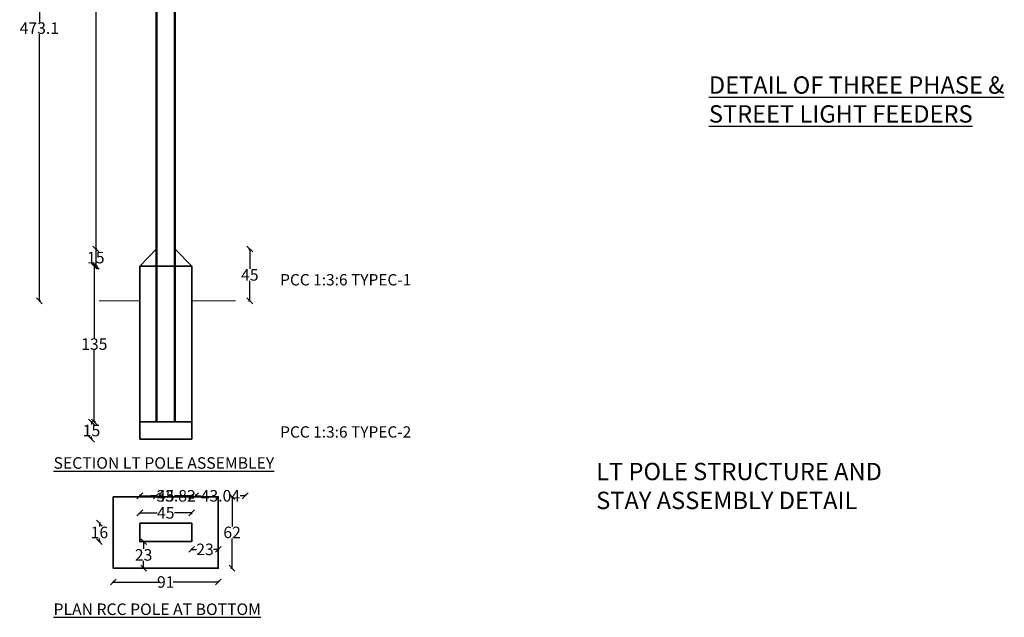
# Model space of a CAD drawing. Units: centimetres. Extents: x -70 to 1009, y -133 to 977.
# Tile 1 of 3: x -66 to 787, y -133 to 385. Entities that reach past the tile are written whole.
import ezdxf

# ---------------------------------------------------------------- set-up
doc = ezdxf.new("R2010")
doc.units = ezdxf.units.CM
doc.header["$MEASUREMENT"] = 0
for name, color, linetype, lineweight in [('C-TOPO', 8, 'Continuous', 18), ('E-ANNO-DIMS', 2, 'Continuous', 18), ('E-ANNO-TEXT', 7, 'Continuous', 25), ('E-POLE', 7, 'Continuous', 50), ('S-FNDN', 1, 'Continuous', 35)]:
    doc.layers.add(name, color=color, linetype=linetype, lineweight=lineweight)
doc.styles.get("Standard").update_dxf_attribs({"font": 'arial.ttf'})
doc.dimstyles.get("Standard").update_dxf_attribs({"dimtxt": 10, "dimasz": 5, "dimexe": 0.1, "dimexo": 0.1, "dimgap": 0.09, "dimtad": 0, "dimtih": 1, "dimtoh": 1, "dimdec": 0, "dimzin": 0, "dimdsep": 46, "dimtxsty": 'Standard', "dimblk": 'OBLIQUE', "dimcen": 0.09, "dimadec": 0, "dimazin": 0, "dimtfac": 1, "dimtdec": 0, "dimtofl": 0, "dimtmove": 0, "dimatfit": 3, "dimfxl": 1, "dimfxlon": 1, "dimtolj": 1, "dimtzin": 0, "dimarcsym": 0})

# ---------------------------------------------------------------- blocks, each defined once
blk = doc.blocks.new('_Oblique')
at = {"color": 0, "linetype": 'ByBlock', "lineweight": -2}
blk.add_line((-0.5, -0.5), (0.5, 0.5), dxfattribs=at)
blk = doc.blocks.new('*D3')
at = {"layer": 'Defpoints', "color": 0, "transparency": 16777216}
for p in [(52.24, 921.22), (-0.04, 171.22), (52.24, 171.22)]:
    blk.add_point(p, dxfattribs=at)
at = {"layer": 'E-ANNO-DIMS', "color": 0, "lineweight": -2, "transparency": 16777216}
for p, q in [((0.96, 921.22), (-0.14, 921.22)), ((-0.04, 921.22), (-0.04, 551.41)), ((-0.04, 171.22), (-0.04, 541.02)), ((0.96, 171.22), (-0.14, 171.22))]:
    blk.add_line(p, q, dxfattribs=at)
at = {"layer": 'E-ANNO-DIMS', "color": 0, "lineweight": -2, "transparency": 16777216, "xscale": 5, "yscale": 5, "zscale": 5}
for p, rotation in [((-0.04, 921.22), 90), ((-0.04, 171.22), 270)]:
    blk.add_blockref('_Oblique', p, dxfattribs=dict(at, rotation=rotation))
at = {"layer": 'E-ANNO-DIMS', "color": 0, "transparency": 16777216, "insert": (-0.04, 546.22), "char_height": 10, "attachment_point": 5}
blk.add_mtext('\\A1;750', dxfattribs=at)
blk = doc.blocks.new('*D4')
at = {"layer": 'Defpoints', "color": 0, "transparency": 16777216}
for p in [(-0.42, 186.22), (52.24, 186.22), (52.75, 171.22)]:
    blk.add_point(p, dxfattribs=at)
at = {"layer": 'E-ANNO-DIMS', "color": 0, "lineweight": -2, "transparency": 16777216}
for p, q in [((0.58, 186.22), (-0.52, 186.22)), ((-0.42, 186.22), (-0.42, 183.91)), ((0.58, 171.22), (-0.52, 171.22)), ((-0.42, 171.22), (-0.42, 173.52))]:
    blk.add_line(p, q, dxfattribs=at)
at = {"layer": 'E-ANNO-DIMS', "color": 0, "lineweight": -2, "transparency": 16777216, "xscale": 5, "yscale": 5, "zscale": 5}
for p, rotation in [((-0.42, 186.22), 90), ((-0.42, 171.22), 270)]:
    blk.add_blockref('_Oblique', p, dxfattribs=dict(at, rotation=rotation))
at = {"layer": 'E-ANNO-DIMS', "color": 0, "transparency": 16777216, "insert": (-0.42, 178.72), "char_height": 10, "attachment_point": 5}
blk.add_mtext('\\A1;15', dxfattribs=at)
blk = doc.blocks.new('*D5')
at = {"layer": 'Defpoints', "color": 0, "transparency": 16777216}
for p in [(37.74, 171.22), (-1.69, 36.22), (37.74, 36.22)]:
    blk.add_point(p, dxfattribs=at)
at = {"layer": 'E-ANNO-DIMS', "color": 0, "lineweight": -2, "transparency": 16777216}
for p, q in [((-0.69, 171.22), (-1.79, 171.22)), ((-1.69, 171.22), (-1.69, 108.91)), ((-1.69, 36.22), (-1.69, 98.52)), ((-0.69, 36.22), (-1.79, 36.22))]:
    blk.add_line(p, q, dxfattribs=at)
at = {"layer": 'E-ANNO-DIMS', "color": 0, "lineweight": -2, "transparency": 16777216, "xscale": 5, "yscale": 5, "zscale": 5}
for p, rotation in [((-1.69, 171.22), 90), ((-1.69, 36.22), 270)]:
    blk.add_blockref('_Oblique', p, dxfattribs=dict(at, rotation=rotation))
at = {"layer": 'E-ANNO-DIMS', "color": 0, "transparency": 16777216, "insert": (-1.69, 103.72), "char_height": 10, "attachment_point": 5}
blk.add_mtext('\\A1;135', dxfattribs=at)
blk = doc.blocks.new('*D6')
at = {"layer": 'Defpoints', "color": 0, "transparency": 16777216}
for p in [(37.74, 36.22), (-4.14, 21.22), (37.74, 21.22)]:
    blk.add_point(p, dxfattribs=at)
at = {"layer": 'E-ANNO-DIMS', "color": 0, "lineweight": -2, "transparency": 16777216}
for p, q in [((-3.14, 36.22), (-4.24, 36.22)), ((-4.14, 36.22), (-4.14, 33.91)), ((-3.14, 21.22), (-4.24, 21.22)), ((-4.14, 21.22), (-4.14, 23.52))]:
    blk.add_line(p, q, dxfattribs=at)
at = {"layer": 'E-ANNO-DIMS', "color": 0, "lineweight": -2, "transparency": 16777216, "xscale": 5, "yscale": 5, "zscale": 5}
for p, rotation in [((-4.14, 36.22), 90), ((-4.14, 21.22), 270)]:
    blk.add_blockref('_Oblique', p, dxfattribs=dict(at, rotation=rotation))
at = {"layer": 'E-ANNO-DIMS', "color": 0, "transparency": 16777216, "insert": (-4.14, 28.72), "char_height": 10, "attachment_point": 5}
blk.add_mtext('\\A1;15', dxfattribs=at)
blk = doc.blocks.new('*D7')
at = {"layer": 'Defpoints', "color": 0, "transparency": 16777216}
for p in [(68.24, 186.22), (133.11, 186.22), (68.24, 141.22)]:
    blk.add_point(p, dxfattribs=at)
at = {"layer": 'E-ANNO-DIMS', "color": 0, "lineweight": -2, "transparency": 16777216}
for p, q in [((132.11, 186.22), (133.21, 186.22)), ((133.11, 186.22), (133.11, 168.89)), ((133.11, 141.22), (133.11, 158.54)), ((132.11, 141.22), (133.21, 141.22))]:
    blk.add_line(p, q, dxfattribs=at)
at = {"layer": 'E-ANNO-DIMS', "color": 0, "lineweight": -2, "transparency": 16777216, "xscale": 5, "yscale": 5, "zscale": 5}
for p, rotation in [((133.11, 186.22), 90), ((133.11, 141.22), 270)]:
    blk.add_blockref('_Oblique', p, dxfattribs=dict(at, rotation=rotation))
at = {"layer": 'E-ANNO-DIMS', "color": 0, "transparency": 16777216, "insert": (133.11, 163.72), "char_height": 10, "attachment_point": 5}
blk.add_mtext('\\A1;45', dxfattribs=at)
blk = doc.blocks.new('*D8')
at = {"layer": 'Defpoints', "color": 0, "transparency": 16777216}
for p in [(82.74, -42.66), (37.74, -51.63), (82.74, -51.63)]:
    blk.add_point(p, dxfattribs=at)
at = {"layer": 'E-ANNO-DIMS', "color": 0, "lineweight": -2, "transparency": 16777216}
for p, q in [((37.74, -43.66), (37.74, -42.56)), ((37.74, -42.66), (52.75, -42.66)), ((82.74, -42.66), (67.73, -42.66)), ((82.74, -43.66), (82.74, -42.56))]:
    blk.add_line(p, q, dxfattribs=at)
at = {"layer": 'E-ANNO-DIMS', "color": 0, "lineweight": -2, "transparency": 16777216, "xscale": 5, "yscale": 5, "zscale": 5, "rotation": 180}
blk.add_blockref('_Oblique', (37.74, -42.66), dxfattribs=at)
at = {"layer": 'E-ANNO-DIMS', "color": 0, "lineweight": -2, "transparency": 16777216, "xscale": 5, "yscale": 5, "zscale": 5}
blk.add_blockref('_Oblique', (82.74, -42.66), dxfattribs=at)
at = {"layer": 'E-ANNO-DIMS', "color": 0, "transparency": 16777216, "insert": (60.24, -42.66), "char_height": 10, "attachment_point": 5}
blk.add_mtext('\\A1;45', dxfattribs=at)
blk = doc.blocks.new('*D9')
at = {"layer": 'Defpoints', "color": 0, "transparency": 16777216}
for p in [(82.74, -67.63), (105.74, -67.63), (105.74, -74.34)]:
    blk.add_point(p, dxfattribs=at)
at = {"layer": 'E-ANNO-DIMS', "color": 0, "lineweight": -2, "transparency": 16777216}
for p, q in [((82.74, -73.34), (82.74, -74.44)), ((82.74, -74.34), (86.9, -74.34)), ((105.74, -74.34), (101.58, -74.34)), ((105.74, -73.34), (105.74, -74.44))]:
    blk.add_line(p, q, dxfattribs=at)
at = {"layer": 'E-ANNO-DIMS', "color": 0, "lineweight": -2, "transparency": 16777216, "xscale": 5, "yscale": 5, "zscale": 5, "rotation": 180}
blk.add_blockref('_Oblique', (82.74, -74.34), dxfattribs=at)
at = {"layer": 'E-ANNO-DIMS', "color": 0, "lineweight": -2, "transparency": 16777216, "xscale": 5, "yscale": 5, "zscale": 5}
blk.add_blockref('_Oblique', (105.74, -74.34), dxfattribs=at)
at = {"layer": 'E-ANNO-DIMS', "color": 0, "transparency": 16777216, "insert": (94.24, -74.34), "char_height": 10, "attachment_point": 5}
blk.add_mtext('\\A1;23', dxfattribs=at)
blk = doc.blocks.new('*D10')
at = {"layer": 'Defpoints', "color": 0, "transparency": 16777216}
for p in [(37.74, -67.63), (37.74, -90.63), (41.03, -90.63)]:
    blk.add_point(p, dxfattribs=at)
at = {"layer": 'E-ANNO-DIMS', "color": 0, "lineweight": -2, "transparency": 16777216}
for p, q in [((40.03, -67.63), (41.13, -67.63)), ((41.03, -67.63), (41.03, -73.93)), ((41.03, -90.63), (41.03, -84.33)), ((40.03, -90.63), (41.13, -90.63))]:
    blk.add_line(p, q, dxfattribs=at)
at = {"layer": 'E-ANNO-DIMS', "color": 0, "lineweight": -2, "transparency": 16777216, "xscale": 5, "yscale": 5, "zscale": 5}
for p, rotation in [((41.03, -67.63), 90), ((41.03, -90.63), 270)]:
    blk.add_blockref('_Oblique', p, dxfattribs=dict(at, rotation=rotation))
at = {"layer": 'E-ANNO-DIMS', "color": 0, "transparency": 16777216, "insert": (41.03, -79.13), "char_height": 10, "attachment_point": 5}
blk.add_mtext('\\A1;23', dxfattribs=at)
blk = doc.blocks.new('*D21')
at = {"layer": 'Defpoints', "color": 0, "transparency": 16777216}
for p in [(14.74, -90.63), (105.74, -90.63), (105.74, -102.63)]:
    blk.add_point(p, dxfattribs=at)
at = {"layer": 'E-ANNO-DIMS', "color": 0, "lineweight": -2, "transparency": 16777216}
for p, q in [((14.74, -101.63), (14.74, -102.73)), ((105.74, -101.63), (105.74, -102.73)), ((14.74, -102.63), (53.95, -102.63)), ((105.74, -102.63), (66.53, -102.63))]:
    blk.add_line(p, q, dxfattribs=at)
at = {"layer": 'E-ANNO-DIMS', "color": 0, "lineweight": -2, "transparency": 16777216, "xscale": 5, "yscale": 5, "zscale": 5, "rotation": 180}
blk.add_blockref('_Oblique', (14.74, -102.63), dxfattribs=at)
at = {"layer": 'E-ANNO-DIMS', "color": 0, "lineweight": -2, "transparency": 16777216, "xscale": 5, "yscale": 5, "zscale": 5}
blk.add_blockref('_Oblique', (105.74, -102.63), dxfattribs=at)
at = {"layer": 'E-ANNO-DIMS', "color": 0, "transparency": 16777216, "insert": (60.24, -102.63), "char_height": 10, "attachment_point": 5}
blk.add_mtext('\\A1;91', dxfattribs=at)
blk = doc.blocks.new('*D22')
at = {"layer": 'Defpoints', "color": 0, "transparency": 16777216}
for p in [(105.74, -28.63), (117.74, -28.63), (105.74, -90.63)]:
    blk.add_point(p, dxfattribs=at)
at = {"layer": 'E-ANNO-DIMS', "color": 0, "lineweight": -2, "transparency": 16777216}
for p, q in [((116.74, -28.63), (117.84, -28.63)), ((117.74, -28.63), (117.74, -54.44)), ((117.74, -90.63), (117.74, -64.83)), ((116.74, -90.63), (117.84, -90.63))]:
    blk.add_line(p, q, dxfattribs=at)
at = {"layer": 'E-ANNO-DIMS', "color": 0, "lineweight": -2, "transparency": 16777216, "xscale": 5, "yscale": 5, "zscale": 5}
for p, rotation in [((117.74, -28.63), 90), ((117.74, -90.63), 270)]:
    blk.add_blockref('_Oblique', p, dxfattribs=dict(at, rotation=rotation))
at = {"layer": 'E-ANNO-DIMS', "color": 0, "transparency": 16777216, "insert": (117.74, -59.63), "char_height": 10, "attachment_point": 5}
blk.add_mtext('\\A1;62', dxfattribs=at)
blk = doc.blocks.new('*D23')
at = {"layer": 'Defpoints', "color": 0, "transparency": 16777216}
for p in [(2.74, -51.63), (37.74, -51.63), (37.74, -67.63)]:
    blk.add_point(p, dxfattribs=at)
at = {"layer": 'E-ANNO-DIMS', "color": 0, "lineweight": -2, "transparency": 16777216}
for p, q in [((3.74, -51.63), (2.64, -51.63)), ((2.74, -51.63), (2.74, -54.44)), ((3.74, -67.63), (2.64, -67.63)), ((2.74, -67.63), (2.74, -64.83))]:
    blk.add_line(p, q, dxfattribs=at)
at = {"layer": 'E-ANNO-DIMS', "color": 0, "lineweight": -2, "transparency": 16777216, "xscale": 5, "yscale": 5, "zscale": 5}
for p, rotation in [((2.74, -51.63), 90), ((2.74, -67.63), 270)]:
    blk.add_blockref('_Oblique', p, dxfattribs=dict(at, rotation=rotation))
at = {"layer": 'E-ANNO-DIMS', "color": 0, "transparency": 16777216, "insert": (2.74, -59.63), "char_height": 10, "attachment_point": 5}
blk.add_mtext('\\A1;16', dxfattribs=at)
blk = doc.blocks.new('*D25')
at = {"layer": 'Defpoints', "color": 0, "transparency": 16777216}
for p in [(37.74, 21.22), (82.74, 21.22), (82.74, -27.88)]:
    blk.add_point(p, dxfattribs=at)
at = {"layer": 'E-ANNO-DIMS', "color": 0, "lineweight": -2, "transparency": 16777216}
for p, q in [((37.74, -26.88), (37.74, -27.98)), ((37.74, -27.88), (52.75, -27.88)), ((82.74, -27.88), (67.73, -27.88)), ((82.74, -26.88), (82.74, -27.98))]:
    blk.add_line(p, q, dxfattribs=at)
at = {"layer": 'E-ANNO-DIMS', "color": 0, "lineweight": -2, "transparency": 16777216, "xscale": 5, "yscale": 5, "zscale": 5, "rotation": 180}
blk.add_blockref('_Oblique', (37.74, -27.88), dxfattribs=at)
at = {"layer": 'E-ANNO-DIMS', "color": 0, "lineweight": -2, "transparency": 16777216, "xscale": 5, "yscale": 5, "zscale": 5}
blk.add_blockref('_Oblique', (82.74, -27.88), dxfattribs=at)
at = {"layer": 'E-ANNO-DIMS', "color": 0, "transparency": 16777216, "insert": (60.24, -27.88), "char_height": 10, "attachment_point": 5}
blk.add_mtext('\\A1;45', dxfattribs=at)
blk = doc.blocks.new('*D34')
at = {"layer": 'Defpoints', "color": 0, "transparency": 16777216}
for p in [(52.24, 614.28), (-49.36, 141.22), (2.39, 141.22)]:
    blk.add_point(p, dxfattribs=at)
at = {"layer": 'E-ANNO-DIMS', "color": 0, "lineweight": -2, "transparency": 16777216}
for p, q in [((-48.36, 614.28), (-49.46, 614.28)), ((-49.36, 614.28), (-49.36, 382.95)), ((-49.36, 141.22), (-49.36, 372.55)), ((-48.36, 141.22), (-49.46, 141.22))]:
    blk.add_line(p, q, dxfattribs=at)
at = {"layer": 'E-ANNO-DIMS', "color": 0, "lineweight": -2, "transparency": 16777216, "xscale": 5, "yscale": 5, "zscale": 5}
for p, rotation in [((-49.36, 614.28), 90), ((-49.36, 141.22), 270)]:
    blk.add_blockref('_Oblique', p, dxfattribs=dict(at, rotation=rotation))
at = {"layer": 'E-ANNO-DIMS', "color": 0, "transparency": 16777216, "insert": (-49.36, 377.75), "char_height": 10, "attachment_point": 5}
blk.add_mtext('\\A1;473.1', dxfattribs=at)
blk = doc.blocks.new('*D35')
at = {"layer": 'Defpoints', "color": 0, "transparency": 16777216}
for p in [(52.23894, 639.625874), (86.058746, 612.513226), (86.058746, -27.884542)]:
    blk.add_point(p, dxfattribs=at)
at = {"layer": 'E-ANNO-DIMS', "color": 0, "lineweight": -2, "transparency": 16777216}
for p, q in [((52.23894, -27.884542), (47.23894, -27.884542)), ((52.23894, -26.884542), (52.23894, -27.984542)), ((86.058746, -26.884542), (86.058746, -27.984542)), ((86.058746, -27.884542), (91.058746, -27.884542))]:
    blk.add_line(p, q, dxfattribs=at)
at = {"layer": 'E-ANNO-DIMS', "color": 0, "lineweight": -2, "transparency": 16777216, "xscale": 5, "yscale": 5, "zscale": 5}
blk.add_blockref('_Oblique', (52.23894, -27.884542), dxfattribs=at)
at = {"layer": 'E-ANNO-DIMS', "color": 0, "lineweight": -2, "transparency": 16777216, "xscale": 5, "yscale": 5, "zscale": 5, "rotation": 180}
blk.add_blockref('_Oblique', (86.058746, -27.884542), dxfattribs=at)
at = {"layer": 'E-ANNO-DIMS', "color": 0, "transparency": 16777216, "insert": (69.148843, -27.884542), "char_height": 10, "attachment_point": 5}
blk.add_mtext('\\A1;33.82', dxfattribs=at)
blk = doc.blocks.new('*D36')
at = {"layer": 'Defpoints', "color": 0, "transparency": 16777216}
for p in [(129.1, 671.11), (86.06, 612.51), (129.1, -27.88)]:
    blk.add_point(p, dxfattribs=at)
at = {"layer": 'E-ANNO-DIMS', "color": 0, "lineweight": -2, "transparency": 16777216}
for p, q in [((86.06, -26.88), (86.06, -27.98)), ((86.06, -27.88), (90.43, -27.88)), ((129.1, -27.88), (124.72, -27.88)), ((129.1, -26.88), (129.1, -27.98))]:
    blk.add_line(p, q, dxfattribs=at)
at = {"layer": 'E-ANNO-DIMS', "color": 0, "lineweight": -2, "transparency": 16777216, "xscale": 5, "yscale": 5, "zscale": 5, "rotation": 180}
blk.add_blockref('_Oblique', (86.06, -27.88), dxfattribs=at)
at = {"layer": 'E-ANNO-DIMS', "color": 0, "lineweight": -2, "transparency": 16777216, "xscale": 5, "yscale": 5, "zscale": 5}
blk.add_blockref('_Oblique', (129.1, -27.88), dxfattribs=at)
at = {"layer": 'E-ANNO-DIMS', "color": 0, "transparency": 16777216, "insert": (107.58, -27.88), "char_height": 10, "attachment_point": 5}
blk.add_mtext('\\A1;43.04', dxfattribs=at)

msp = doc.modelspace()

# ---------------------------------------------------------------- linework, layer by layer
at = {"layer": 'C-TOPO'}
for p, q in [((37.7389, 141.2155), (2.3883, 141.2155)), ((82.7389, 141.2155), (120.6906, 141.2155))]:
    msp.add_line(p, q, dxfattribs=at)
at = {"layer": 'E-POLE'}
for p, q in [((52.2389, 171.2155), (52.2389, 921.2155)), ((68.2389, 171.2155), (68.2389, 921.2155)), ((68.2389, 186.2155), (68.2389, 141.2155)), ((52.2389, 36.2155), (52.2389, 171.2155)), ((68.2389, 36.2155), (68.2389, 171.2155))]:
    msp.add_line(p, q, dxfattribs=at)
at = {"layer": 'S-FNDN'}
for p, q in [((52.2389, 186.2155), (37.7389, 171.2155)), ((68.2389, 186.2155), (82.7389, 171.2155)), ((82.7389, 171.2155), (37.7389, 171.2155)), ((37.7389, 171.2155), (37.7389, 36.2155)), ((82.7389, 36.2155), (82.7389, 171.2155)), ((82.7389, 36.2155), (37.7389, 36.2155)), ((37.7389, 36.2155), (37.7389, 21.2155)), ((82.7389, 21.2155), (82.7389, 36.2155)), ((37.7389, 21.2155), (82.7389, 21.2155))]:
    msp.add_line(p, q, dxfattribs=at)
for points in [[(14.7389, -28.6341), (105.7389, -28.6341), (105.7389, -90.6341), (14.7389, -90.6341)], [(37.7389, -51.6341), (82.7389, -51.6341), (82.7389, -67.6341), (37.7389, -67.6341)]]:
    msp.add_lwpolyline(points, close=True, dxfattribs=at)

# ---------------------------------------------------------------- texts
at = {"layer": 'E-ANNO-TEXT', "attachment_point": 1}
for s, width, gutter_width, insert, char_height in [('{\\fArial|b1|i0|c0|p34;\\LDETAIL OF THREE PHASE & \\PSTREET LIGHT FEEDERS}', 528.222344, 2.9584, (531.0806, 335.9284), 15.039493), ('PCC 1:3:6 TYPEC-1', 351.223506, 1.9671, (159.4237, 164.4233), 9.835469), ('PCC 1:3:6 TYPEC-2', 351.223506, 1.9671, (159.4237, 32.4228), 9.835469), ('{\\fArial|b1|i0|c0|p34;\\LSECTION LT POLE ASSEMBLEY}', 351.223506, 1.9671, (-37.0364, 5.6056), 10), ('{\\fArial|b1|i1|c0|p34;LT POLE STRUCTURE AND \\PSTAY ASSEMBLY DETAIL}', 528.222344, 2.9584, (433.3816, 0.7244), 15.039493), ('{\\fArial|b1|i0|c0|p34;\\LPLAN RCC POLE AT BOTTOM}', 351.223506, 1.9671, (-37.0364, -121.2531), 10)]:
    msp.add_mtext_dynamic_manual_height_columns(s, width=width, gutter_width=gutter_width, heights=[0], dxfattribs=dict(at, insert=insert, char_height=char_height))

# ---------------------------------------------------------------- dimensions: what is measured, and where the dimension line sits
at = {"layer": 'E-ANNO-DIMS'}
for base, p1, p2, override, picture, middle in [((-0.0426, 171.2155), (52.2389, 921.2155), (52.2389, 171.2155), {"dimclrd": 0, "dimclre": 0, "dimclrt": 0}, '*D3', (-0.0426, 546.2155)), ((-49.3611, 141.2155), (52.2389, 614.2808), (2.3883, 141.2155), {"dimdec": 1, "dimlfac": 1, "dimrnd": 0, "dimzin": 0, "dimdsep": 46, "dimlunit": 2}, '*D34', (-49.3611, 377.7481)), ((-0.4226, 186.2155), (52.7476, 171.2155), (52.2389, 186.2155), {"dimclrd": 0, "dimclre": 0, "dimclrt": 0}, '*D4', (-0.4226, 178.7155)), ((133.1124, 186.2155), (68.2389, 141.2155), (68.2389, 186.2155), {"dimclrd": 0, "dimclre": 0, "dimclrt": 0}, '*D7', (133.1124, 163.7155)), ((-1.6873, 36.2155), (37.7389, 171.2155), (37.7389, 36.2155), {"dimclrd": 0, "dimclre": 0, "dimclrt": 0}, '*D5', (-1.6873, 103.7155)), ((-4.1353, 21.2155), (37.7389, 36.2155), (37.7389, 21.2155), {"dimclrd": 0, "dimclre": 0, "dimclrt": 0}, '*D6', (-4.1353, 28.7155)), ((117.7389, -28.6341), (105.7389, -90.6341), (105.7389, -28.6341), {"dimdec": 0, "dimlfac": 1, "dimrnd": 0, "dimzin": 0, "dimdsep": 46, "dimlunit": 2}, '*D22', (117.7389, -59.6341)), ((2.7389, -51.6341), (37.7389, -67.6341), (37.7389, -51.6341), {"dimdec": 0, "dimlfac": 1, "dimrnd": 0, "dimzin": 0, "dimdsep": 46, "dimlunit": 2}, '*D23', (2.7389, -59.6341)), ((41.0282, -90.6341), (37.7389, -67.6341), (37.7389, -90.6341), {"dimclrd": 0, "dimclre": 0, "dimclrt": 0}, '*D10', (41.0282, -79.1341))]:
    dim = msp.add_linear_dim(base=base, p1=p1, p2=p2, angle=90, dimstyle='Standard', override=override, dxfattribs=at)
    dim.commit()
    dim.dimension.update_dxf_attribs({"geometry": picture, "text_midpoint": middle})
for base, p1, p2, override, picture, middle in [((129.0952, -27.8845), (86.0587, 612.5132), (129.0952, 671.1109), {"dimdec": 2, "dimlfac": 1, "dimrnd": 0, "dimzin": 0, "dimdsep": 46, "dimlunit": 2}, '*D36', (107.577, -27.8845)), ((86.0587, -27.8845), (52.2389, 639.6259), (86.0587, 612.5132), {"dimdec": 2, "dimlfac": 1, "dimrnd": 0, "dimzin": 0, "dimdsep": 46, "dimlunit": 2}, '*D35', (69.1488, -27.8845)), ((82.7389, -27.8845), (37.7389, 21.2155), (82.7389, 21.2155), {"dimdec": 0, "dimlfac": 1, "dimrnd": 0, "dimzin": 0, "dimdsep": 46, "dimlunit": 2}, '*D25', (60.2389, -27.8845)), ((82.7389, -42.6552), (37.7389, -51.6341), (82.7389, -51.6341), {"dimclrd": 0, "dimclre": 0, "dimclrt": 0}, '*D8', (60.2389, -42.6552)), ((105.7389, -74.3387), (82.7389, -67.6341), (105.7389, -67.6341), {"dimclrd": 0, "dimclre": 0, "dimclrt": 0}, '*D9', (94.2389, -74.3387)), ((105.7389, -102.6341), (14.7389, -90.6341), (105.7389, -90.6341), {"dimdec": 0, "dimlfac": 1, "dimrnd": 0, "dimzin": 0, "dimdsep": 46, "dimlunit": 2}, '*D21', (60.2389, -102.6341))]:
    dim = msp.add_linear_dim(base=base, p1=p1, p2=p2, dimstyle='Standard', override=override, dxfattribs=at)
    dim.commit()
    dim.dimension.update_dxf_attribs({"geometry": picture, "text_midpoint": middle})

doc.saveas('drawing.dxf')
